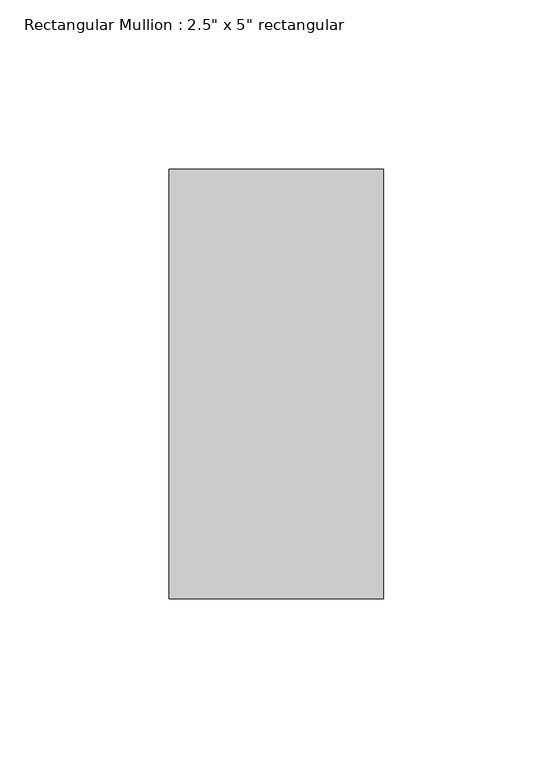
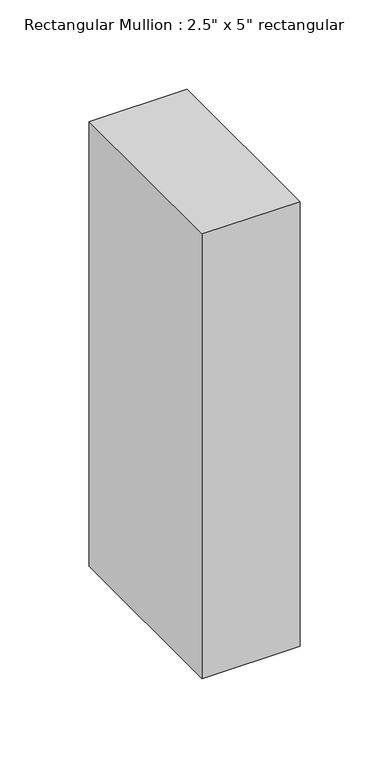
"""IFC4 building model written with IfcOpenShell, lengths in millimetres: member geometry."""

from ifc_helpers import new_model, si_unit, frame, origin, place, context, project, spatial, polyline, outline, extrude, source, transform, mapped, element, save


def member_75d1e245(model_context):
    return source(origin(), model_context, "Body", "SweptSolid", [
        extrude(outline(polyline([(31.75, 63.5), (31.75, -63.5), (-31.75, -63.5), (-31.75, 63.5), (31.75, 63.5)])), frame((0.0, 0.0, -304.8), z_axis=(0.0, 0.0, 1.0), x_axis=(1.0, 0.0, 0.0)), (0.0, 0.0, 1.0), 304.8),
    ])


if __name__ == "__main__":
    model = new_model("IFC4")
    model_context = context("Model", 3, world=origin())
    ifc_project = project(units=[si_unit("LENGTHUNIT", "METRE", prefix="MILLI")], contexts=[model_context])
    site = spatial("IfcSite", under=ifc_project)
    building = spatial("IfcBuilding", under=site)
    placement = place(None, origin())
    member_shape = member_75d1e245(model_context)
    element("IfcMember", 1, ObjectType="Rectangular Mullion : 2.5\" x 5\" rectangular", at=placement, inside=building, context=model_context, shape_type="MappedRepresentation", body=[
        mapped(member_shape, transform((0.0, 0.0, 0.0), x_axis=(1.0, 0.0, 0.0), y_axis=(0.0, 1.0, 0.0), z_axis=(0.0, 0.0, 1.0))),
    ])
    save(model, "model.ifc")

# Revit data of these elements
# Type "Rectangular Mullion : 2.5\" x 5\" rectangular"
#   built-in parameter 1007304 = 0.416667 (stored number, unit not read)
#   built-in parameter 1007301 = 0.104167 (stored number, unit not read)
#   built-in parameter 1007300 = 0.104167 (stored number, unit not read)
# Element 1 (IfcMember, "Rectangular Mullion : 2.5\" x 5\" rectangular")
#   Materials on its faces: "Aluminum"
# Materials
#   "Aluminum": class "Metal", colour RGB 247 247 247, transparency 0, Description = "Aluminum 6061", Cost = 0
